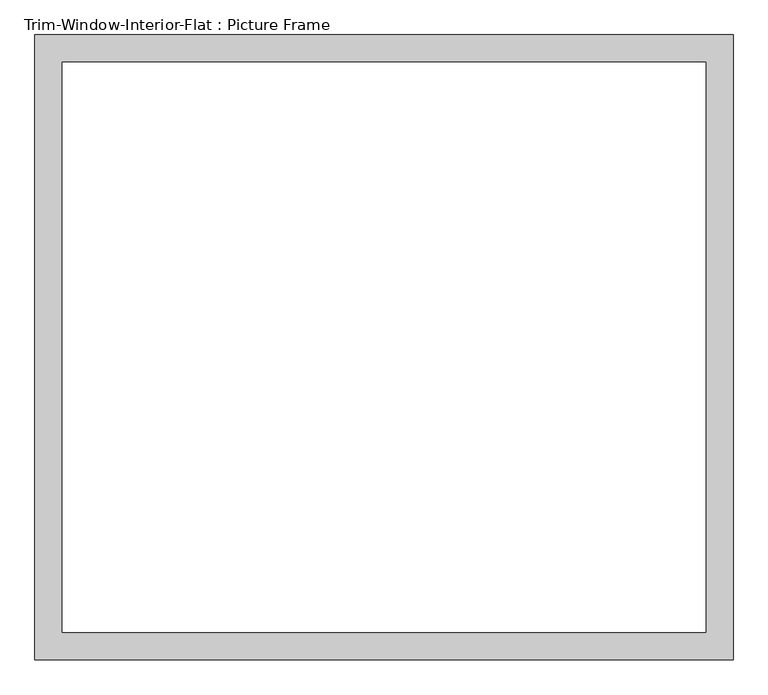
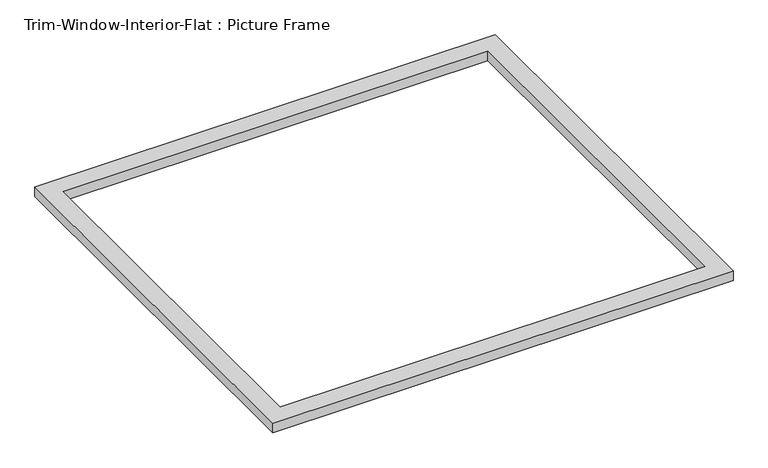
"""IFC4 building model written with IfcOpenShell, lengths in millimetres: proxy geometry, Trim-Window-Interior-Flat : Picture Frame."""

from ifc_helpers import new_model, si_unit, origin, origin_with_axes, place, context, project, spatial, polyline, outline, extrude, source, transform, mapped, element, save


def trim_window_interior_flat_picture_frame_3949a48f(model_context):
    return source(origin(), model_context, "Body", "SweptSolid", [
        extrude(outline(polyline([(730.25, 44.45), (730.25, -1263.65), (-730.25, -1263.65), (-730.25, 44.45), (730.25, 44.45)]), holes=[polyline([(673.1, -12.7), (-673.1, -12.7), (-673.1, -1206.5), (673.1, -1206.5), (673.1, -12.7)])]), origin_with_axes(), (0.0, 0.0, 1.0), 31.75),
    ])


if __name__ == "__main__":
    model = new_model("IFC4")
    model_context = context("Model", 3, world=origin())
    ifc_project = project(units=[si_unit("LENGTHUNIT", "METRE", prefix="MILLI")], contexts=[model_context])
    site = spatial("IfcSite", under=ifc_project)
    building = spatial("IfcBuilding", under=site)
    placement = place(None, origin())
    trim_window_interior_flat_picture_frame_shape = trim_window_interior_flat_picture_frame_3949a48f(model_context)
    element("IfcBuildingElementProxy", 1, Name="Trim-Window-Interior-Flat : Picture Frame", ObjectType="Trim-Window-Interior-Flat : Picture Frame", at=placement, inside=building, context=model_context, shape_type="MappedRepresentation", body=[
        mapped(trim_window_interior_flat_picture_frame_shape, transform((0.0, 0.0, 0.0), x_axis=(1.0, 0.0, 0.0), y_axis=(0.0, 1.0, 0.0), z_axis=(0.0, 0.0, 1.0))),
    ])
    save(model, "model.ifc")

# Revit data of these elements
# Type "Trim-Window-Interior-Flat : Picture Frame"
#   Trim Thickness_Picture Frame = 0' - 1 1/4"
#   Trim Width = 0' - 2 1/4"
#   Trim Thickness_with Sill = 0' - 0 3/4"
#   Sill Thickness = 0' - 1 1/4"
#   Opening Width [instance default] = 2' - 0"
#   Opening Height [instance default] = 3' - 0"
#   Default Elevation = 4' - 0"
#   Sill = no
#   Picture Frame = yes
#   Trim Material [instance default] = none
# Element 1 (IfcBuildingElementProxy, "Trim-Window-Interior-Flat : Picture Frame")
#   Opening Width = 4' - 6"
#   Opening Height = 4' - 0"
#   Trim Material = Wood - Stained
#   Materials on its faces: "Wood - Stained"
# Materials
#   "Wood - Stained": class "Wood", colour RGB 224 178 126, transparency 0, Cost = 0
